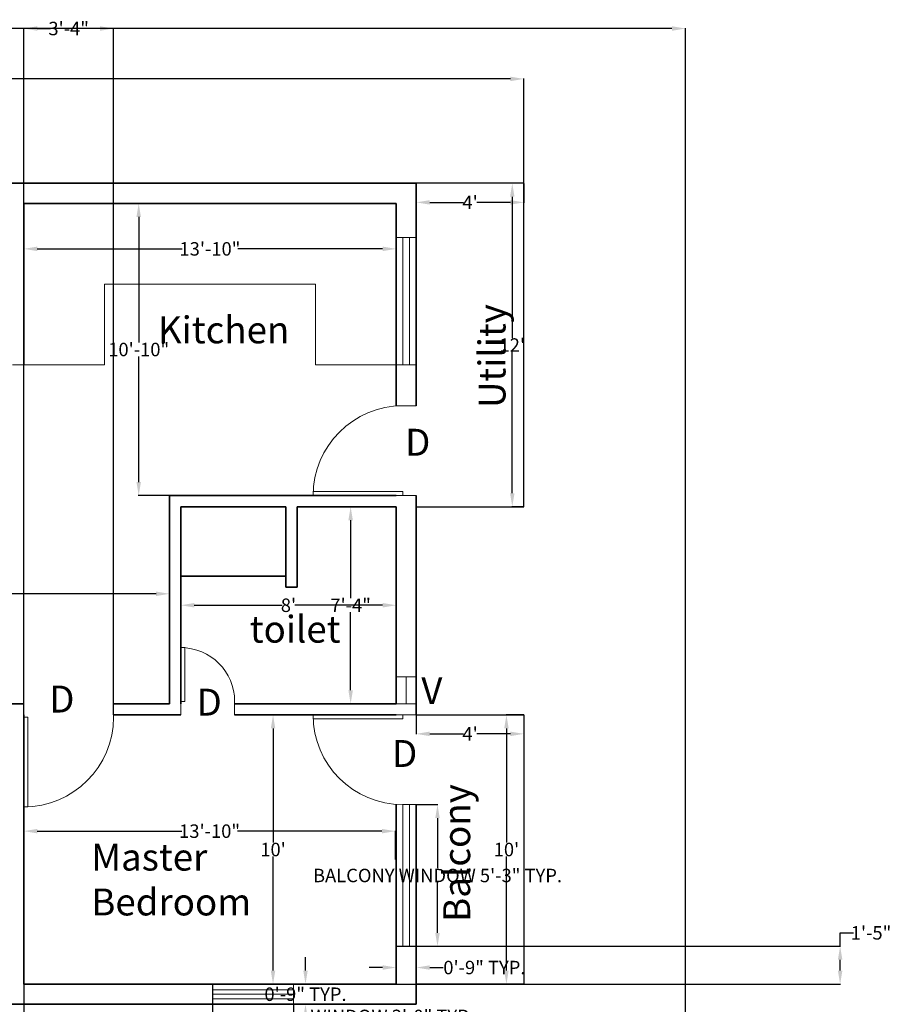
# Model space of a CAD drawing. Units: inches. Extents: x 1936 to 2761, y 1431 to 2889.
# Tile 6 of 6: x 2372 to 2761, y 2451 to 2889. Entities that reach past the tile are written whole.
import ezdxf

# ---------------------------------------------------------------- set-up
doc = ezdxf.new("R2010")
doc.units = ezdxf.units.IN
doc.header["$MEASUREMENT"] = 0
for name, color, linetype, lineweight in [('A-ANNO-DIMS', 172, 'Continuous', 13), ('A-ANNO-TEXT', 50, 'Continuous', 18), ('A-AREA-IDEN', 50, 'Continuous', 18), ('A-FLOR-EDGE', 4, 'Continuous', 25), ('A-FLOR-FIXT', 8, 'Continuous', 18), ('A-GLAZ', 3, 'Continuous', 18), ('A-WALL', 4, 'Continuous', 35), ('doors', 10, 'Continuous', 18)]:
    doc.layers.add(name, color=color, linetype=linetype, lineweight=lineweight)
doc.styles.get("Standard").update_dxf_attribs({"font": 'arial.ttf'})
doc.dimstyles.get("Standard").update_dxf_attribs({"dimtxt": 6, "dimasz": 6, "dimexe": 0.18, "dimexo": 0.0625, "dimgap": 0.09, "dimtad": 0, "dimtih": 1, "dimtoh": 1, "dimdec": 0, "dimzin": 0, "dimdsep": 46, "dimlunit": 3, "dimtxsty": 'Standard', "dimcen": 0.09, "dimadec": 0, "dimazin": 0, "dimtfac": 1, "dimtdec": 0, "dimtofl": 0, "dimtmove": 0, "dimatfit": 3, "dimfxl": 1, "dimtolj": 1, "dimtzin": 0, "dimarcsym": 0})

# ---------------------------------------------------------------- blocks, each defined once
blk = doc.blocks.new('*U2')
for p, q in [((0, 0), (0, 6)), ((40, 0), (40, 6))]:
    blk.add_line(p, q)
blk.add_lwpolyline([(0, 0), (0, -40), (1.75, -40), (1.75, 0)], close=True)
blk.add_arc((0, 0), 40, 270, 360)
blk = doc.blocks.new('*U3')
for p, q in [((0, 0), (0, -6)), ((24, 0), (24, -6))]:
    blk.add_line(p, q)
blk.add_lwpolyline([(0, 0), (0, 24), (1.75, 24), (1.75, 0)], close=True)
blk.add_arc((0, 0), 24, 0, 90)
blk = doc.blocks.new('*U5')
for p, q in [((0, 0), (0, -6)), ((40, 0), (40, -6))]:
    blk.add_line(p, q)
blk.add_lwpolyline([(0, 0), (0, 40), (1.75, 40), (1.75, 0)], close=True)
blk.add_arc((0, 0), 40, 0, 90)
blk = doc.blocks.new('*D10')
at = {"layer": 'A-ANNO-DIMS', "color": 0, "lineweight": -2, "transparency": 16777216}
for p, q in [((2249.01, 2633.61), (2249.01, 2633.73)), ((2439.01, 2633.61), (2439.01, 2633.73)), ((2255.01, 2633.55), (2331.56, 2633.55)), ((2433.01, 2633.55), (2356.45, 2633.55))]:
    blk.add_line(p, q, dxfattribs=at)
at = {"layer": 'A-ANNO-DIMS', "color": 0, "transparency": 16777216}
for points in [[(2255.01, 2634.55), (2255.01, 2632.55), (2249.01, 2633.55)], [(2433.01, 2634.55), (2433.01, 2632.55), (2439.01, 2633.55)]]:
    blk.add_solid(points, dxfattribs=at)
at = {"layer": 'Defpoints', "color": 0, "transparency": 16777216}
for p in [(2249.01, 2633.55), (2439.01, 2633.55), (2439.01, 2633.55)]:
    blk.add_point(p, dxfattribs=at)
at = {"layer": 'A-ANNO-DIMS', "color": 0, "transparency": 16777216, "insert": (2344.01, 2633.55), "char_height": 6, "attachment_point": 5}
blk.add_mtext('\\A1;15\'-10"', dxfattribs=at)
blk = doc.blocks.new('*D12')
at = {"layer": 'A-ANNO-DIMS', "color": 0, "lineweight": -2, "transparency": 16777216}
for p, q in [((2374.01, 2787.38), (2374.01, 2787.5)), ((2380.01, 2787.32), (2444.56, 2787.32)), ((2534.01, 2787.32), (2469.45, 2787.32)), ((2540.01, 2787.38), (2540.01, 2787.5))]:
    blk.add_line(p, q, dxfattribs=at)
at = {"layer": 'A-ANNO-DIMS', "color": 0, "transparency": 16777216}
for points in [[(2380.01, 2788.32), (2380.01, 2786.32), (2374.01, 2787.32)], [(2534.01, 2788.32), (2534.01, 2786.32), (2540.01, 2787.32)]]:
    blk.add_solid(points, dxfattribs=at)
at = {"layer": 'Defpoints', "color": 0, "transparency": 16777216}
for p in [(2374.01, 2787.32), (2540.01, 2787.32), (2540.01, 2787.32)]:
    blk.add_point(p, dxfattribs=at)
at = {"layer": 'A-ANNO-DIMS', "color": 0, "transparency": 16777216, "insert": (2457.01, 2787.32), "char_height": 6, "attachment_point": 5}
blk.add_mtext('\\A1;13\'-10"', dxfattribs=at)
blk = doc.blocks.new('*D13')
at = {"layer": 'A-ANNO-DIMS', "color": 0, "lineweight": -2, "transparency": 16777216}
for p, q in [((2485.38, 2807.55), (2425.06, 2807.55)), ((2425.24, 2801.55), (2425.24, 2745.61)), ((2425.24, 2683.36), (2425.24, 2739.3)), ((2489.44, 2677.36), (2425.06, 2677.36))]:
    blk.add_line(p, q, dxfattribs=at)
at = {"layer": 'A-ANNO-DIMS', "color": 0, "transparency": 16777216}
for points in [[(2424.24, 2801.55), (2426.24, 2801.55), (2425.24, 2807.55)], [(2424.24, 2683.36), (2426.24, 2683.36), (2425.24, 2677.36)]]:
    blk.add_solid(points, dxfattribs=at)
at = {"layer": 'Defpoints', "color": 0, "transparency": 16777216}
for p in [(2485.44, 2807.55), (2425.24, 2677.36), (2489.51, 2677.36)]:
    blk.add_point(p, dxfattribs=at)
at = {"layer": 'A-ANNO-DIMS', "color": 0, "transparency": 16777216, "insert": (2425.24, 2742.45), "char_height": 6, "attachment_point": 5}
blk.add_mtext('\\A1;10\'-10"', dxfattribs=at)
blk = doc.blocks.new('*D14')
at = {"layer": 'A-ANNO-DIMS', "color": 0, "lineweight": -2, "transparency": 16777216}
for p, q in [((2444.01, 2628.52), (2444.01, 2628.63)), ((2450.01, 2628.45), (2489.15, 2628.45)), ((2534.01, 2628.45), (2494.86, 2628.45)), ((2540.01, 2628.52), (2540.01, 2628.63))]:
    blk.add_line(p, q, dxfattribs=at)
at = {"layer": 'A-ANNO-DIMS', "color": 0, "transparency": 16777216}
for points in [[(2450.01, 2629.45), (2450.01, 2627.45), (2444.01, 2628.45)], [(2534.01, 2629.45), (2534.01, 2627.45), (2540.01, 2628.45)]]:
    blk.add_solid(points, dxfattribs=at)
at = {"layer": 'Defpoints', "color": 0, "transparency": 16777216}
for p in [(2444.01, 2628.45), (2540.01, 2628.45), (2540.01, 2628.45)]:
    blk.add_point(p, dxfattribs=at)
at = {"layer": 'A-ANNO-DIMS', "color": 0, "transparency": 16777216, "insert": (2492.01, 2628.45), "char_height": 6, "attachment_point": 5}
blk.add_mtext("\\A1;8'", dxfattribs=at)
blk = doc.blocks.new('*D15')
at = {"layer": 'A-ANNO-DIMS', "color": 0, "lineweight": -2, "transparency": 16777216}
for p, q in [((2518.02, 2672.36), (2519.92, 2672.36)), ((2519.74, 2666.36), (2519.74, 2631.54)), ((2519.74, 2590.55), (2519.74, 2625.36)), ((2518.02, 2584.55), (2519.92, 2584.55))]:
    blk.add_line(p, q, dxfattribs=at)
at = {"layer": 'A-ANNO-DIMS', "color": 0, "transparency": 16777216}
for points in [[(2518.74, 2666.36), (2520.74, 2666.36), (2519.74, 2672.36)], [(2518.74, 2590.55), (2520.74, 2590.55), (2519.74, 2584.55)]]:
    blk.add_solid(points, dxfattribs=at)
at = {"layer": 'Defpoints', "color": 0, "transparency": 16777216}
for p in [(2517.96, 2672.36), (2517.96, 2584.55), (2519.74, 2584.55)]:
    blk.add_point(p, dxfattribs=at)
at = {"layer": 'A-ANNO-DIMS', "color": 0, "transparency": 16777216, "insert": (2519.74, 2628.45), "char_height": 6, "attachment_point": 5}
blk.add_mtext('\\A1;7\'-4"', dxfattribs=at)
blk = doc.blocks.new('*D24')
at = {"layer": 'A-ANNO-DIMS', "color": 0, "lineweight": -2, "transparency": 16777216}
for p, q in [((2374.01, 2515.1), (2374.01, 2527.92)), ((2380.01, 2527.74), (2444.41, 2527.74)), ((2533.69, 2527.74), (2469.29, 2527.74)), ((2539.69, 2515.1), (2539.69, 2527.92))]:
    blk.add_line(p, q, dxfattribs=at)
at = {"layer": 'A-ANNO-DIMS', "color": 0, "transparency": 16777216}
for points in [[(2380.01, 2528.74), (2380.01, 2526.74), (2374.01, 2527.74)], [(2533.69, 2528.74), (2533.69, 2526.74), (2539.69, 2527.74)]]:
    blk.add_solid(points, dxfattribs=at)
at = {"layer": 'Defpoints', "color": 0, "transparency": 16777216}
for p in [(2374.01, 2527.74), (2374.01, 2515.04), (2539.69, 2515.04)]:
    blk.add_point(p, dxfattribs=at)
at = {"layer": 'A-ANNO-DIMS', "color": 0, "transparency": 16777216, "insert": (2456.85, 2527.74), "char_height": 6, "attachment_point": 5}
blk.add_mtext('\\A1;13\'-10"', dxfattribs=at)
blk = doc.blocks.new('*D25')
at = {"layer": 'A-ANNO-DIMS', "color": 0, "lineweight": -2, "transparency": 16777216}
for p, q in [((2480.34, 2579.55), (2485.32, 2579.55)), ((2485.14, 2573.55), (2485.14, 2522.7)), ((2485.14, 2465.55), (2485.14, 2516.4)), ((2480.34, 2459.55), (2485.32, 2459.55))]:
    blk.add_line(p, q, dxfattribs=at)
at = {"layer": 'A-ANNO-DIMS', "color": 0, "transparency": 16777216}
for points in [[(2484.14, 2573.55), (2486.14, 2573.55), (2485.14, 2579.55)], [(2484.14, 2465.55), (2486.14, 2465.55), (2485.14, 2459.55)]]:
    blk.add_solid(points, dxfattribs=at)
at = {"layer": 'Defpoints', "color": 0, "transparency": 16777216}
for p in [(2480.28, 2579.55), (2485.14, 2579.55), (2480.28, 2459.55)]:
    blk.add_point(p, dxfattribs=at)
at = {"layer": 'A-ANNO-DIMS', "color": 0, "transparency": 16777216, "insert": (2485.14, 2519.55), "char_height": 6, "attachment_point": 5}
blk.add_mtext("\\A1;10'", dxfattribs=at)
blk = doc.blocks.new('*D28')
at = {"layer": 'A-ANNO-DIMS', "color": 0, "lineweight": -2, "transparency": 16777216}
for p, q in [((2549.01, 2816.49), (2549.01, 2807.86)), ((2597.01, 2816.49), (2597.01, 2807.86)), ((2555.01, 2808.04), (2570.03, 2808.04)), ((2591.01, 2808.04), (2575.98, 2808.04))]:
    blk.add_line(p, q, dxfattribs=at)
at = {"layer": 'A-ANNO-DIMS', "color": 0, "transparency": 16777216}
for points in [[(2555.01, 2809.04), (2555.01, 2807.04), (2549.01, 2808.04)], [(2591.01, 2809.04), (2591.01, 2807.04), (2597.01, 2808.04)]]:
    blk.add_solid(points, dxfattribs=at)
at = {"layer": 'Defpoints', "color": 0, "transparency": 16777216}
for p in [(2549.01, 2816.55), (2597.01, 2816.55), (2597.01, 2808.04)]:
    blk.add_point(p, dxfattribs=at)
at = {"layer": 'A-ANNO-DIMS', "color": 0, "transparency": 16777216, "insert": (2573.01, 2808.04), "char_height": 6, "attachment_point": 5}
blk.add_mtext("\\A1;4'", dxfattribs=at)
blk = doc.blocks.new('*D29')
at = {"layer": 'A-ANNO-DIMS', "color": 0, "lineweight": -2, "transparency": 16777216}
for p, q in [((2596.94, 2816.55), (2591.63, 2816.55)), ((2591.81, 2810.55), (2591.81, 2747.56)), ((2591.81, 2678.36), (2591.81, 2741.35)), ((2596.94, 2672.36), (2591.63, 2672.36))]:
    blk.add_line(p, q, dxfattribs=at)
at = {"layer": 'A-ANNO-DIMS', "color": 0, "transparency": 16777216}
for points in [[(2590.81, 2810.55), (2592.81, 2810.55), (2591.81, 2816.55)], [(2590.81, 2678.36), (2592.81, 2678.36), (2591.81, 2672.36)]]:
    blk.add_solid(points, dxfattribs=at)
at = {"layer": 'Defpoints', "color": 0, "transparency": 16777216}
for p in [(2597.01, 2816.55), (2591.81, 2672.36), (2597.01, 2672.36)]:
    blk.add_point(p, dxfattribs=at)
at = {"layer": 'A-ANNO-DIMS', "color": 0, "transparency": 16777216, "insert": (2591.81, 2744.45), "char_height": 6, "attachment_point": 5}
blk.add_mtext("\\A1;12'", dxfattribs=at)
blk = doc.blocks.new('*D30')
at = {"layer": 'A-ANNO-DIMS', "color": 0, "lineweight": -2, "transparency": 16777216}
for p, q in [((2549.01, 2579.49), (2549.01, 2570.93)), ((2597.01, 2579.49), (2597.01, 2570.93)), ((2555.01, 2571.11), (2570.03, 2571.11)), ((2591.01, 2571.11), (2575.98, 2571.11))]:
    blk.add_line(p, q, dxfattribs=at)
at = {"layer": 'A-ANNO-DIMS', "color": 0, "transparency": 16777216}
for points in [[(2555.01, 2572.11), (2555.01, 2570.11), (2549.01, 2571.11)], [(2591.01, 2572.11), (2591.01, 2570.11), (2597.01, 2571.11)]]:
    blk.add_solid(points, dxfattribs=at)
at = {"layer": 'Defpoints', "color": 0, "transparency": 16777216}
for p in [(2549.01, 2579.55), (2597.01, 2579.55), (2597.01, 2571.11)]:
    blk.add_point(p, dxfattribs=at)
at = {"layer": 'A-ANNO-DIMS', "color": 0, "transparency": 16777216, "insert": (2573.01, 2571.11), "char_height": 6, "attachment_point": 5}
blk.add_mtext("\\A1;4'", dxfattribs=at)
blk = doc.blocks.new('*D31')
at = {"layer": 'A-ANNO-DIMS', "color": 0, "lineweight": -2, "transparency": 16777216}
for p, q in [((2596.94, 2579.55), (2589.03, 2579.55)), ((2589.21, 2573.55), (2589.21, 2522.7)), ((2589.21, 2465.55), (2589.21, 2516.4)), ((2596.94, 2459.55), (2589.03, 2459.55))]:
    blk.add_line(p, q, dxfattribs=at)
at = {"layer": 'A-ANNO-DIMS', "color": 0, "transparency": 16777216}
for points in [[(2588.21, 2573.55), (2590.21, 2573.55), (2589.21, 2579.55)], [(2588.21, 2465.55), (2590.21, 2465.55), (2589.21, 2459.55)]]:
    blk.add_solid(points, dxfattribs=at)
at = {"layer": 'Defpoints', "color": 0, "transparency": 16777216}
for p in [(2597.01, 2579.55), (2589.21, 2459.55), (2597.01, 2459.55)]:
    blk.add_point(p, dxfattribs=at)
at = {"layer": 'A-ANNO-DIMS', "color": 0, "transparency": 16777216, "insert": (2589.21, 2519.55), "char_height": 6, "attachment_point": 5}
blk.add_mtext("\\A1;10'", dxfattribs=at)
blk = doc.blocks.new('*D80')
at = {"layer": 'A-ANNO-DIMS', "color": 0, "lineweight": -2, "transparency": 16777216}
for p, q in [((2021.01, 2816.61), (2021.01, 2863.26)), ((2027.01, 2863.08), (2298.49, 2863.08)), ((2591.01, 2863.08), (2319.52, 2863.08)), ((2597.01, 2816.61), (2597.01, 2863.26))]:
    blk.add_line(p, q, dxfattribs=at)
at = {"layer": 'A-ANNO-DIMS', "color": 0, "transparency": 16777216}
for points in [[(2027.01, 2864.08), (2027.01, 2862.08), (2021.01, 2863.08)], [(2591.01, 2864.08), (2591.01, 2862.08), (2597.01, 2863.08)]]:
    blk.add_solid(points, dxfattribs=at)
at = {"layer": 'Defpoints', "color": 0, "transparency": 16777216}
for p in [(2021.01, 2863.08), (2021.01, 2816.55), (2597.01, 2816.55)]:
    blk.add_point(p, dxfattribs=at)
at = {"layer": 'A-ANNO-DIMS', "color": 0, "transparency": 16777216, "insert": (2309.01, 2863.08), "char_height": 6, "attachment_point": 5}
blk.add_mtext("\\A1;{\\H2x;48'}", dxfattribs=at)
blk = doc.blocks.new('WIN-36')
for p, q in [((0, 9), (0, 0)), ((36, 9), (36, 0)), ((36, 6.5), (0, 6.5)), ((36, 4.5), (0, 4.5)), ((36, 2.5), (0, 2.5))]:
    blk.add_line(p, q)
blk = doc.blocks.new('VENT-12')
for p, q in [((0, 0), (0, 9)), ((12, 0), (12, 9)), ((0, 4.5), (12, 4.5))]:
    blk.add_line(p, q)
blk = doc.blocks.new('WIN-KITCHEN')
for p, q in [((0, 56.83), (9, 56.83)), ((3, 56.83), (3, 0)), ((6, 56.83), (6, 0)), ((0, 0), (9, 0))]:
    blk.add_line(p, q)
blk = doc.blocks.new('WIN-BALCONY')
for p, q in [((3, 63.14), (3, 0)), ((6, 63.14), (6, 0)), ((0, 0), (9, 0))]:
    blk.add_line(p, q)
blk = doc.blocks.new('COUNTER-KITCHEN-U')
for p, q in [((41, 36), (41, 0)), ((41, 36), (135, 36)), ((135, 36), (135, 0)), ((0, 0), (41, 0)), ((135, 0), (171, 0))]:
    blk.add_line(p, q)
blk = doc.blocks.new('BATH-PARTITION')
for p, q in [((0, 35.9), (46.9, 35.9)), ((0, 5), (0, 35.9)), ((46.9, 35.9), (46.9, 0)), ((51.9, 35.9), (51.9, 0)), ((46.9, 5), (0, 5)), ((51.9, 0), (46.9, 0))]:
    blk.add_line(p, q)
blk = doc.blocks.new('*D87')
at = {"layer": 'A-ANNO-DIMS', "color": 0, "lineweight": -2, "transparency": 16777216}
for p, q in [((2458.21, 2450.49), (2458.21, 2444.97)), ((2494.21, 2450.49), (2494.21, 2444.97)), ((2464.21, 2445.15), (2488.21, 2445.15)), ((2494.21, 2445.15), (2500.21, 2445.15))]:
    blk.add_line(p, q, dxfattribs=at)
at = {"layer": 'A-ANNO-DIMS', "color": 0, "transparency": 16777216}
for points in [[(2464.21, 2446.15), (2464.21, 2444.15), (2458.21, 2445.15)], [(2488.21, 2446.15), (2488.21, 2444.15), (2494.21, 2445.15)]]:
    blk.add_solid(points, dxfattribs=at)
at = {"layer": 'Defpoints', "color": 0, "transparency": 16777216}
for p in [(2458.21, 2450.55), (2494.21, 2450.55), (2494.21, 2445.15)]:
    blk.add_point(p, dxfattribs=at)
at = {"layer": 'A-ANNO-DIMS', "color": 0, "transparency": 16777216, "insert": (2538.26, 2445.15), "char_height": 6, "attachment_point": 5}
blk.add_mtext('\\A1;WINDOW 3\'-0" TYP.', dxfattribs=at)
blk = doc.blocks.new('*D88')
at = {"layer": 'A-ANNO-DIMS', "color": 0, "lineweight": -2, "transparency": 16777216}
for p, q in [((2499.61, 2465.55), (2499.61, 2471.55)), ((2494.27, 2459.55), (2499.79, 2459.55)), ((2494.27, 2450.55), (2499.79, 2450.55)), ((2499.61, 2444.55), (2499.61, 2438.55))]:
    blk.add_line(p, q, dxfattribs=at)
at = {"layer": 'A-ANNO-DIMS', "color": 0, "transparency": 16777216}
for points in [[(2498.61, 2465.55), (2500.61, 2465.55), (2499.61, 2459.55)], [(2498.61, 2444.55), (2500.61, 2444.55), (2499.61, 2450.55)]]:
    blk.add_solid(points, dxfattribs=at)
at = {"layer": 'Defpoints', "color": 0, "transparency": 16777216}
for p in [(2494.21, 2459.55), (2499.61, 2459.55), (2494.21, 2450.55)]:
    blk.add_point(p, dxfattribs=at)
at = {"layer": 'A-ANNO-DIMS', "color": 0, "transparency": 16777216, "insert": (2499.61, 2455.05), "char_height": 6, "attachment_point": 5}
blk.add_mtext('\\A1;0\'-9" TYP.', dxfattribs=at)
blk = doc.blocks.new('*D97')
at = {"layer": 'A-ANNO-DIMS', "color": 0, "lineweight": -2, "transparency": 16777216}
for p, q in [((2549.07, 2539.55), (2558.66, 2539.55)), ((2558.48, 2533.55), (2558.48, 2511.18)), ((2558.48, 2482.41), (2558.48, 2504.78)), ((2549.07, 2476.41), (2558.66, 2476.41))]:
    blk.add_line(p, q, dxfattribs=at)
at = {"layer": 'A-ANNO-DIMS', "color": 0, "transparency": 16777216}
for points in [[(2557.48, 2533.55), (2559.48, 2533.55), (2558.48, 2539.55)], [(2557.48, 2482.41), (2559.48, 2482.41), (2558.48, 2476.41)]]:
    blk.add_solid(points, dxfattribs=at)
at = {"layer": 'Defpoints', "color": 0, "transparency": 16777216}
for p in [(2549.01, 2539.55), (2558.48, 2539.55), (2549.01, 2476.41)]:
    blk.add_point(p, dxfattribs=at)
at = {"layer": 'A-ANNO-DIMS', "color": 0, "transparency": 16777216, "insert": (2558.48, 2507.98), "char_height": 6, "attachment_point": 5}
blk.add_mtext('\\A1;BALCONY WINDOW 5\'-3" TYP.', dxfattribs=at)
blk = doc.blocks.new('*D98')
at = {"layer": 'A-ANNO-DIMS', "color": 0, "lineweight": -2, "transparency": 16777216}
for p, q in [((2540.01, 2476.35), (2540.01, 2466.76)), ((2549.01, 2476.35), (2549.01, 2466.76)), ((2534.01, 2466.94), (2528.01, 2466.94)), ((2555.01, 2466.94), (2561.01, 2466.94))]:
    blk.add_line(p, q, dxfattribs=at)
at = {"layer": 'A-ANNO-DIMS', "color": 0, "transparency": 16777216}
for points in [[(2534.01, 2467.94), (2534.01, 2465.94), (2540.01, 2466.94)], [(2555.01, 2467.94), (2555.01, 2465.94), (2549.01, 2466.94)]]:
    blk.add_solid(points, dxfattribs=at)
at = {"layer": 'Defpoints', "color": 0, "transparency": 16777216}
for p in [(2540.01, 2476.41), (2549.01, 2476.41), (2549.01, 2466.94)]:
    blk.add_point(p, dxfattribs=at)
at = {"layer": 'A-ANNO-DIMS', "color": 0, "transparency": 16777216, "insert": (2579.38, 2466.94), "char_height": 6, "attachment_point": 5}
blk.add_mtext('\\A1;0\'-9" TYP.', dxfattribs=at)
blk = doc.blocks.new('*D99')
at = {"layer": 'A-ANNO-DIMS', "color": 0, "lineweight": -2, "transparency": 16777216}
for p, q in [((2021.01, 2816.61), (2021.01, 2885.73)), ((2027.01, 2885.55), (2334.61, 2885.55)), ((2663.01, 2885.55), (2355.4, 2885.55)), ((2669.01, 2360.61), (2669.01, 2885.73))]:
    blk.add_line(p, q, dxfattribs=at)
at = {"layer": 'A-ANNO-DIMS', "color": 0, "transparency": 16777216}
for points in [[(2027.01, 2886.55), (2027.01, 2884.55), (2021.01, 2885.55)], [(2663.01, 2886.55), (2663.01, 2884.55), (2669.01, 2885.55)]]:
    blk.add_solid(points, dxfattribs=at)
at = {"layer": 'Defpoints', "color": 0, "transparency": 16777216}
for p in [(2669.01, 2885.55), (2021.01, 2816.55), (2669.01, 2360.55)]:
    blk.add_point(p, dxfattribs=at)
at = {"layer": 'A-ANNO-DIMS', "color": 0, "transparency": 16777216, "insert": (2345.01, 2885.55), "char_height": 6, "attachment_point": 5}
blk.add_mtext('\\A1;54\'-0"', dxfattribs=at)
blk = doc.blocks.new('*D109')
at = {"layer": 'A-ANNO-DIMS', "color": 0, "lineweight": -2, "transparency": 16777216}
for p, q in [((2374.01, 2579.61), (2374.01, 2885.73)), ((2380.01, 2885.55), (2385.94, 2885.55)), ((2408.01, 2885.55), (2402.07, 2885.55)), ((2414.01, 2579.61), (2414.01, 2885.73))]:
    blk.add_line(p, q, dxfattribs=at)
at = {"layer": 'A-ANNO-DIMS', "color": 0, "transparency": 16777216}
for points in [[(2380.01, 2886.55), (2380.01, 2884.55), (2374.01, 2885.55)], [(2408.01, 2886.55), (2408.01, 2884.55), (2414.01, 2885.55)]]:
    blk.add_solid(points, dxfattribs=at)
at = {"layer": 'Defpoints', "color": 0, "transparency": 16777216}
for p in [(2414.01, 2885.55), (2374.01, 2579.55), (2414.01, 2579.55)]:
    blk.add_point(p, dxfattribs=at)
at = {"layer": 'A-ANNO-DIMS', "color": 0, "transparency": 16777216, "insert": (2394.01, 2885.55), "char_height": 6, "attachment_point": 5}
blk.add_mtext('\\A1;3\'-4"', dxfattribs=at)
blk = doc.blocks.new('*D112')
at = {"layer": 'A-ANNO-DIMS', "color": 0, "lineweight": -2, "transparency": 16777216}
for p, q in [((2374.01, 2459.49), (2374.01, 1439.37)), ((2458.21, 2459.49), (2458.21, 1439.37)), ((2380.01, 1439.55), (2408.07, 1439.55)), ((2452.21, 1439.55), (2424.15, 1439.55))]:
    blk.add_line(p, q, dxfattribs=at)
at = {"layer": 'A-ANNO-DIMS', "color": 0, "transparency": 16777216}
for points in [[(2380.01, 1440.55), (2380.01, 1438.55), (2374.01, 1439.55)], [(2452.21, 1440.55), (2452.21, 1438.55), (2458.21, 1439.55)]]:
    blk.add_solid(points, dxfattribs=at)
at = {"layer": 'Defpoints', "color": 0, "transparency": 16777216}
for p in [(2374.01, 2459.55), (2458.21, 2459.55), (2458.21, 1439.55)]:
    blk.add_point(p, dxfattribs=at)
at = {"layer": 'A-ANNO-DIMS', "color": 0, "transparency": 16777216, "insert": (2416.11, 1439.55), "char_height": 6, "attachment_point": 5}
blk.add_mtext('\\A1;7\'-0"', dxfattribs=at)
blk = doc.blocks.new('*D113')
at = {"layer": 'A-ANNO-DIMS', "color": 0, "lineweight": -2, "transparency": 16777216}
for p, q in [((2738.01, 2476.41), (2738.01, 2482.41)), ((2738.01, 2482.41), (2744.01, 2482.41)), ((2540.07, 2476.41), (2738.19, 2476.41)), ((2738.01, 2465.55), (2738.01, 2470.41)), ((2540.07, 2459.55), (2738.19, 2459.55))]:
    blk.add_line(p, q, dxfattribs=at)
at = {"layer": 'A-ANNO-DIMS', "color": 0, "transparency": 16777216}
for points in [[(2737.01, 2470.41), (2739.01, 2470.41), (2738.01, 2476.41)], [(2737.01, 2465.55), (2739.01, 2465.55), (2738.01, 2459.55)]]:
    blk.add_solid(points, dxfattribs=at)
at = {"layer": 'Defpoints', "color": 0, "transparency": 16777216}
for p in [(2540.01, 2476.41), (2738.01, 2476.41), (2540.01, 2459.55)]:
    blk.add_point(p, dxfattribs=at)
at = {"layer": 'A-ANNO-DIMS', "color": 0, "transparency": 16777216, "insert": (2751.79, 2482.41), "char_height": 6, "attachment_point": 5}
blk.add_mtext('\\A1;1\'-5"', dxfattribs=at)

msp = doc.modelspace()

# ---------------------------------------------------------------- linework, layer by layer
at = {"layer": 'A-FLOR-EDGE'}
for p, q in [((2597.01, 2816.55), (2549.01, 2816.55)), ((2597.01, 2672.36), (2597.01, 2816.55)), ((2549.01, 2672.36), (2597.01, 2672.36)), ((2549.01, 2579.55), (2597.01, 2579.55)), ((2597.01, 2579.55), (2597.01, 2459.55)), ((2597.01, 2459.55), (2549.01, 2459.55))]:
    msp.add_line(p, q, dxfattribs=at)
at = {"layer": 'A-WALL'}
for p, q in [((2069.01, 2816.55), (2549.01, 2816.55)), ((2549.01, 2816.55), (2549.01, 2717.36)), ((2374.01, 2807.55), (2374.01, 2735.55)), ((2374.01, 2807.55), (2540.01, 2807.55)), ((2540.01, 2807.55), (2540.01, 2717.36)), ((2439.01, 2677.36), (2439.01, 2584.55)), ((2439.01, 2677.36), (2540.01, 2677.36)), ((2549.01, 2677.36), (2549.01, 2579.55)), ((2444.01, 2672.36), (2444.01, 2584.55)), ((2444.01, 2672.36), (2490.9, 2672.36)), ((2495.9, 2672.36), (2540.01, 2672.36)), ((2540.01, 2672.36), (2540.01, 2584.55)), ((2374.01, 2584.55), (2289.01, 2584.55)), ((2439.01, 2584.55), (2414.01, 2584.55)), ((2540.01, 2584.55), (2468.01, 2584.55)), ((2374.01, 2579.55), (2374.01, 2459.55)), ((2444.01, 2579.55), (2414.01, 2579.55)), ((2540.01, 2579.55), (2468.01, 2579.55)), ((2540.01, 2539.66), (2540.01, 2459.55)), ((2549.01, 2539.55), (2549.01, 2450.55)), ((2540.01, 2459.55), (2374.01, 2459.55)), ((2549.01, 2450.55), (2118.01, 2450.55))]:
    msp.add_line(p, q, dxfattribs=at)
at = {"layer": 'doors'}
for p, q in [((2540.01, 2717.36), (2549.01, 2717.36)), ((2540.01, 2677.36), (2549.01, 2677.36)), ((2374.01, 2584.55), (2374.01, 2579.55)), ((2414.01, 2584.55), (2414.01, 2579.55)), ((2444.01, 2584.55), (2444.01, 2579.55)), ((2468.01, 2584.55), (2468.01, 2579.55)), ((2540.01, 2579.55), (2549.01, 2579.55))]:
    msp.add_line(p, q, dxfattribs=at)

# ---------------------------------------------------------------- block references
at = {"layer": 'A-FLOR-FIXT'}
msp.add_blockref('COUNTER-KITCHEN-U', (2369.01, 2735.55), dxfattribs=at)
at = {"layer": 'A-GLAZ'}
for name, p in [('WIN-KITCHEN', (2540.01, 2735.55)), ('WIN-BALCONY', (2540.01, 2476.41)), ('WIN-36', (2458.21, 2450.55))]:
    msp.add_blockref(name, p, dxfattribs=at)
at = {"layer": 'A-GLAZ', "rotation": 270.0000000000007}
msp.add_blockref('VENT-12', (2540.01, 2596.55), dxfattribs=at)
at = {"layer": 'A-WALL'}
msp.add_blockref('BATH-PARTITION', (2444.01, 2636.46), dxfattribs=at)
at = {"layer": 'doors', "rotation": 90}
msp.add_blockref('*U5', (2543.01, 2677.36), dxfattribs=at)
at = {"layer": 'doors'}
for name, p in [('*U3', (2444.01, 2585.55)), ('*U2', (2374.01, 2578.55))]:
    msp.add_blockref(name, p, dxfattribs=at)
at = {"layer": 'doors', "xscale": -1, "rotation": 90}
msp.add_blockref('*U5', (2543.01, 2579.55), dxfattribs=at)

# ---------------------------------------------------------------- texts
at = {"layer": 'A-ANNO-TEXT', "char_height": 12, "attachment_point": 1}
for s, width, heights, insert in [('D', 28.2371, [0.2], (2544.03, 2707.11)), ('V', 13.1151, [0], (2551.24, 2596.37)), ('D', 28.2371, [0.2], (2385.33, 2592.61)), ('D', 28.2371, [0.2], (2451.04, 2591.24)), ('D', 28.2371, [0.2], (2538.2, 2568.35))]:
    msp.add_mtext_dynamic_manual_height_columns(s, width=width, gutter_width=1, heights=heights, dxfattribs=dict(at, insert=insert))
at = {"layer": 'A-AREA-IDEN', "char_height": 12, "attachment_point": 1, "rotation": 90}
for s, insert in [('Utility', (2576.79, 2716.35)), ('Balcony', (2561.04, 2487.28))]:
    msp.add_mtext_dynamic_manual_height_columns(s, width=55.7076, gutter_width=1, heights=[0], dxfattribs=dict(at, insert=insert))
at = {"layer": 'A-AREA-IDEN', "char_height": 12, "attachment_point": 1}
for s, insert in [('Kitchen', (2433.82, 2757.2)), ('toilet', (2474.76, 2623.77)), ('Master Bedroom', (2404.08, 2522.17))]:
    msp.add_mtext_dynamic_manual_height_columns(s, width=55.7076, gutter_width=1, heights=[0], dxfattribs=dict(at, insert=insert))

# ---------------------------------------------------------------- dimensions: what is measured, and where the dimension line sits
at = {"layer": 'A-ANNO-DIMS'}
for base, p1, p2, override, picture, middle in [((2669.01, 2885.55), (2021.01, 2816.55), (2669.01, 2360.55), {"dimdec": 1, "dimlfac": 1, "dimrnd": 0, "dimzin": 1, "dimdsep": 46, "dimlunit": 4, "dimfrac": 2}, '*D99', (2345.01, 2885.55)), ((2414.01, 2885.55), (2374.01, 2579.55), (2414.01, 2579.55), {"dimdec": 1, "dimlfac": 1, "dimrnd": 0, "dimzin": 1, "dimdsep": 46, "dimlunit": 4, "dimfrac": 2}, '*D109', (2394.01, 2885.55)), ((2597.01, 2808.04), (2549.01, 2816.55), (2597.01, 2816.55), {"dimclrd": 0, "dimclre": 0, "dimclrt": 0}, '*D28', (2573.01, 2808.04)), ((2540.01, 2787.32), (2374.01, 2787.32), (2540.01, 2787.32), {"dimclrd": 0, "dimclre": 0, "dimclrt": 0}, '*D12', (2457.01, 2787.32)), ((2439.01, 2633.55), (2249.01, 2633.55), (2439.01, 2633.55), {"dimclrd": 0, "dimclre": 0, "dimclrt": 0}, '*D10', (2344.01, 2633.55)), ((2540.01, 2628.45), (2444.01, 2628.45), (2540.01, 2628.45), {"dimclrd": 0, "dimclre": 0, "dimclrt": 0}, '*D14', (2492.01, 2628.45)), ((2597.01, 2571.11), (2549.01, 2579.55), (2597.01, 2579.55), {"dimclrd": 0, "dimclre": 0, "dimclrt": 0}, '*D30', (2573.01, 2571.11)), ((2374.01, 2527.74), (2539.69, 2515.04), (2374.01, 2515.04), {"dimclrd": 0, "dimclre": 0, "dimclrt": 0}, '*D24', (2456.85, 2527.74)), ((2458.21, 1439.55), (2374.01, 2459.55), (2458.21, 2459.55), {"dimdec": 1, "dimlfac": 1, "dimrnd": 0, "dimzin": 1, "dimdsep": 46, "dimlunit": 4, "dimfrac": 2}, '*D112', (2416.11, 1439.55))]:
    dim = msp.add_linear_dim(base=base, p1=p1, p2=p2, dimstyle='Standard', override=override, dxfattribs=at)
    dim.commit()
    dim.dimension.update_dxf_attribs({"geometry": picture, "text_midpoint": middle})
for base, p1, p2, text, override, picture, middle in [((2021.01, 2863.08), (2597.01, 2816.55), (2021.01, 2816.55), '{\\H2x;<>}', {"dimclrd": 0, "dimclre": 0, "dimclrt": 0}, '*D80', (2309.01, 2863.08)), ((2549.01, 2466.94), (2540.01, 2476.41), (2549.01, 2476.41), '<> TYP.', {"dimdec": 1, "dimlfac": 1, "dimrnd": 0, "dimzin": 1, "dimdsep": 46, "dimlunit": 4, "dimfrac": 2}, '*D98', (2579.38, 2466.94)), ((2494.21, 2445.15), (2458.21, 2450.55), (2494.21, 2450.55), 'WINDOW <> TYP.', {"dimdec": 1, "dimlfac": 1, "dimrnd": 0, "dimzin": 1, "dimdsep": 46, "dimlunit": 4, "dimfrac": 2}, '*D87', (2538.26, 2445.15))]:
    dim = msp.add_linear_dim(base=base, p1=p1, p2=p2, text=text, dimstyle='Standard', override=override, dxfattribs=at)
    dim.commit()
    dim.dimension.update_dxf_attribs({"geometry": picture, "text_midpoint": middle})
for base, p1, p2, override, picture, middle in [((2591.81, 2672.36), (2597.01, 2816.55), (2597.01, 2672.36), {"dimclrd": 0, "dimclre": 0, "dimclrt": 0}, '*D29', (2591.81, 2744.45)), ((2425.24, 2677.36), (2485.44, 2807.55), (2489.51, 2677.36), {"dimclrd": 0, "dimclre": 0, "dimclrt": 0}, '*D13', (2425.24, 2742.45)), ((2519.74, 2584.55), (2517.96, 2672.36), (2517.96, 2584.55), {"dimclrd": 0, "dimclre": 0, "dimclrt": 0}, '*D15', (2519.74, 2628.45)), ((2485.14, 2579.55), (2480.28, 2459.55), (2480.28, 2579.55), {"dimclrd": 0, "dimclre": 0, "dimclrt": 0}, '*D25', (2485.14, 2519.55)), ((2589.21, 2459.55), (2597.01, 2579.55), (2597.01, 2459.55), {"dimclrd": 0, "dimclre": 0, "dimclrt": 0}, '*D31', (2589.21, 2519.55)), ((2738.01, 2476.41), (2540.01, 2459.55), (2540.01, 2476.41), {"dimdec": 1, "dimlfac": 1, "dimrnd": 0, "dimzin": 1, "dimdsep": 46, "dimlunit": 4, "dimfrac": 2}, '*D113', (2751.79, 2482.41))]:
    dim = msp.add_linear_dim(base=base, p1=p1, p2=p2, angle=90, dimstyle='Standard', override=override, dxfattribs=at)
    dim.commit()
    dim.dimension.update_dxf_attribs({"geometry": picture, "text_midpoint": middle})
for base, p1, p2, text, picture, middle in [((2558.48, 2539.55), (2549.01, 2476.41), (2549.01, 2539.55), 'BALCONY WINDOW <> TYP.', '*D97', (2558.48, 2507.98)), ((2499.61, 2459.55), (2494.21, 2450.55), (2494.21, 2459.55), '<> TYP.', '*D88', (2499.61, 2455.05))]:
    dim = msp.add_linear_dim(base=base, p1=p1, p2=p2, angle=90, text=text, dimstyle='Standard', override={"dimdec": 1, "dimlfac": 1, "dimrnd": 0, "dimzin": 1, "dimdsep": 46, "dimlunit": 4, "dimfrac": 2}, dxfattribs=at)
    dim.commit()
    dim.dimension.update_dxf_attribs({"geometry": picture, "text_midpoint": middle})

doc.saveas('drawing.dxf')
